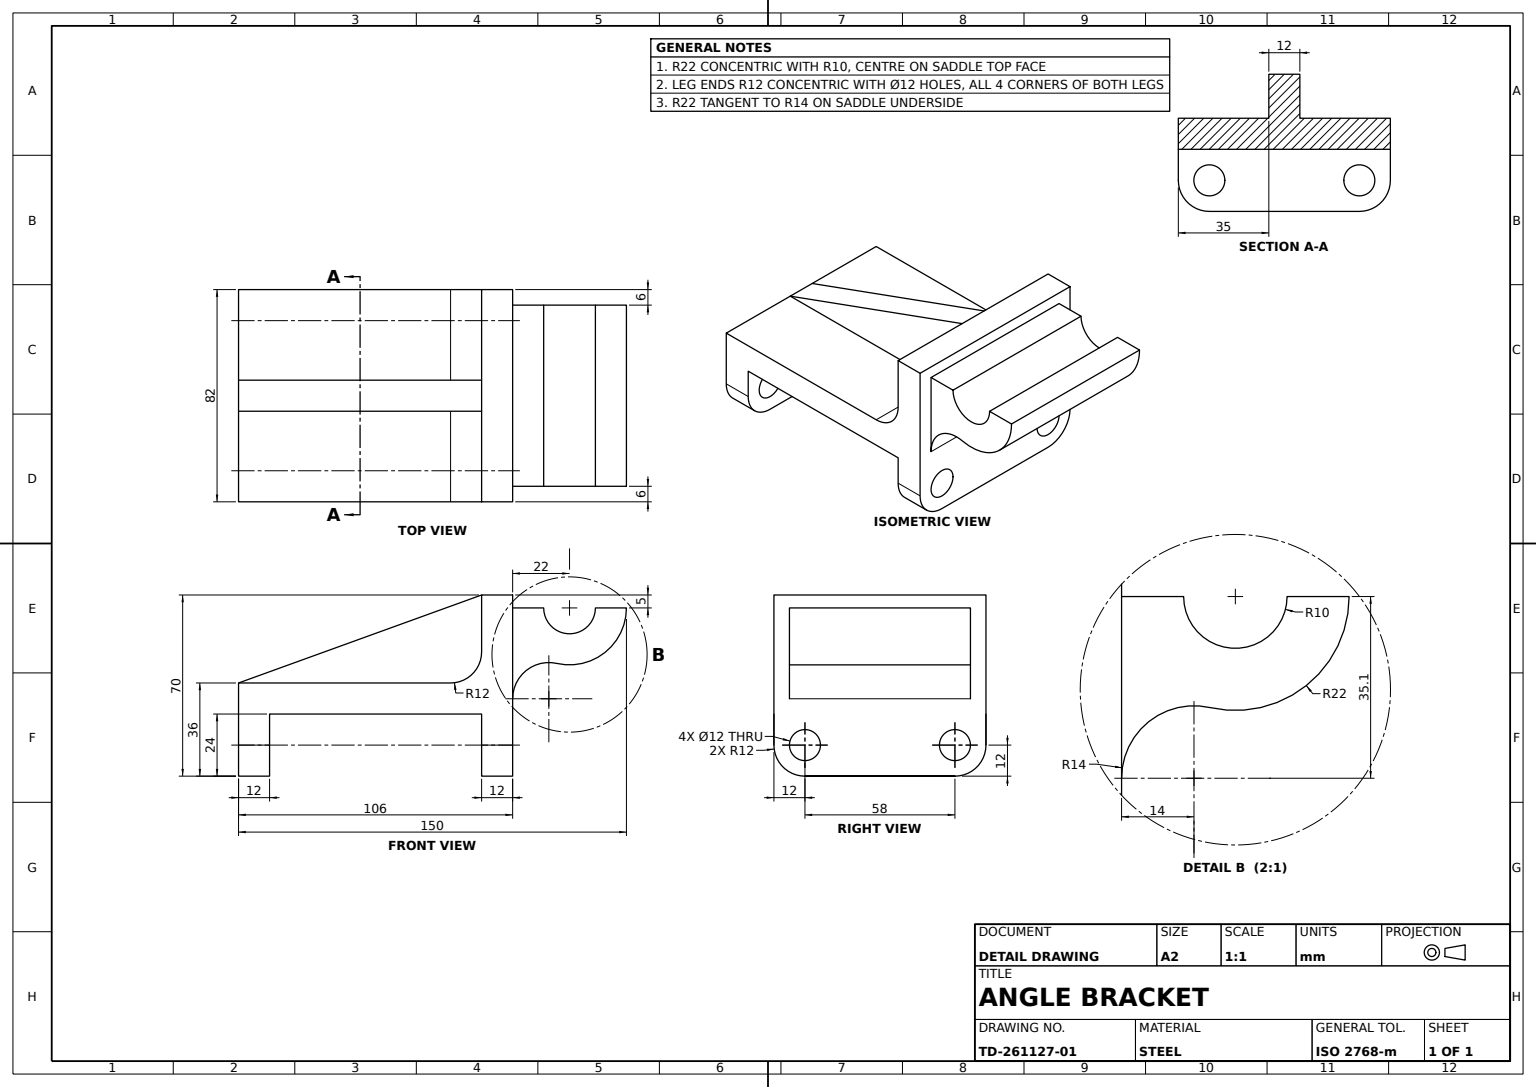
SolidWorks part; units mm, degrees
material "Plain Carbon Steel"
ref_plane "Front Plane" through (0, 0, 0) normal (0, 0, 1) x (1, 0, 0)
ref_plane "Top Plane" through (0, 0, 0) normal (0, 1, 0) x (1, 0, 0)
ref_plane "Right Plane" through (0, 0, 0) normal (1, 0, 0) x (0, 0, -1)
sketch "Base Profile Sketch" plane through (0, 0, 0) normal (0, 1, 0) x (1, 0, 0)
  line L1 (-53, -41) -> (53, -41)
  line L2 (-53, -41) -> (-53, 41)
  line L3 (-53, 41) -> (53, 41)
  line L4 (53, -41) -> (53, 41)
  line L5 (-53, -41) -> (53, 41) construction
  line L6 (-53, 41) -> (53, -41) construction
  point P0 (0, 0)
  dimension "D1" = 106
  dimension "D2" = 82
extrude "Base Block" add sketch "Base Profile Sketch" along normal blind 36
sketch "Underside Channel Sketch" plane through (0, 0, 41) normal (0, 0, 1) x (1, 0, 0)
  line L0 (-53, 0) -> (53, 0) construction
  line L1 (-41, 0) -> (41, 0)
  line L2 (-41, 0) -> (-41, 24)
  line L3 (-41, 24) -> (41, 24)
  line L4 (41, 0) -> (41, 24)
  line L5 (-53, 36) -> (53, 36) construction
  dimension "D1" = 12
  dimension "D2" = 12
  dimension "D3" = 12
extrude "Underside Channel Cut" cut sketch "Underside Channel Sketch" against normal through all
fillet "Base Corner Fillets R12" radius 12 4 edges at (47, 0, -41) (47, 0, 41) (-47, 0, -41) (-47, 0, 41)
sketch "Mounting Holes Sketch" plane through (-53, 0, 0) normal (-1, 0, 0) x (0, 0, 1)
  circle A0 centre (29, 12) radius 6
  circle A1 centre (-29, 12) radius 6
  dimension "D1" = 12
  dimension "D2" = 12
extrude "Mounting Holes Ø12" cut sketch "Mounting Holes Sketch" against normal through all
sketch "Upright Plate Sketch" plane through (0, 0, 41) normal (0, 0, 1) x (1, 0, 0)
  line L1 (53, 36) -> (41, 36)
  line L2 (53, 36) -> (53, 70)
  line L3 (53, 70) -> (41, 70)
  line L4 (41, 36) -> (41, 70)
  dimension "D1" = 12
  dimension "D2" = 34
extrude "Upright Plate" add sketch "Upright Plate Sketch" against normal blind 82
ref_plane "Plane1" through (0, 0, 35) normal (0, 0, 1) x (1, 0, 0)
sketch "Saddle Block Sketch" plane through (0, 0, 35) normal (0, 0, 1) x (1, 0, 0)
  line L0 (53, 65) -> (97, 65)
  line L1 (53, 70) -> (53, 12) construction
  line L2 (53, 29.9001) -> (53, 65)
  arc A0 (70.1111, 43.5501) -> (97, 65) centre (75, 65) ccw
  arc A1 (70.1111, 43.5501) -> (53, 29.9001) centre (67, 29.9001) ccw
  dimension "D3" = 14
  dimension "D1" = 44
  dimension "D2" = 5
extrude "Saddle Block" add sketch "Saddle Block Sketch" against normal blind 70
sketch "Saddle Groove Sketch" plane through (0, 0, 35) normal (0, 0, 1) x (1, 0, 0)
  line L0 (97, 65) -> (53, 65) construction
  circle A0 centre (75, 65) radius 10
  dimension "D1" = 20
extrude "Saddle Groove Ø20" cut sketch "Saddle Groove Sketch" against normal blind 82
ref_plane "Plane2" through (0, 0, 0) normal (0, 0, 1) x (1, 0, 0)
sketch "Reinforcing Rib Sketch" plane through (0, 0, 0) normal (0, 0, 1) x (1, 0, 0)
  line L0 (41, 70) -> (-53, 36)
rib "Reinforcing Rib" sketch "Reinforcing Rib Sketch" sketch "Reinforcing Rib Sketch" thickness 12 extrusion direction parallel to sketch draft on no parameters "D1"=12
fillet "Upright Plate Fillets R12" radius 12 2 edges at (41, 36, -23.5) (41, 36, 23.5)
